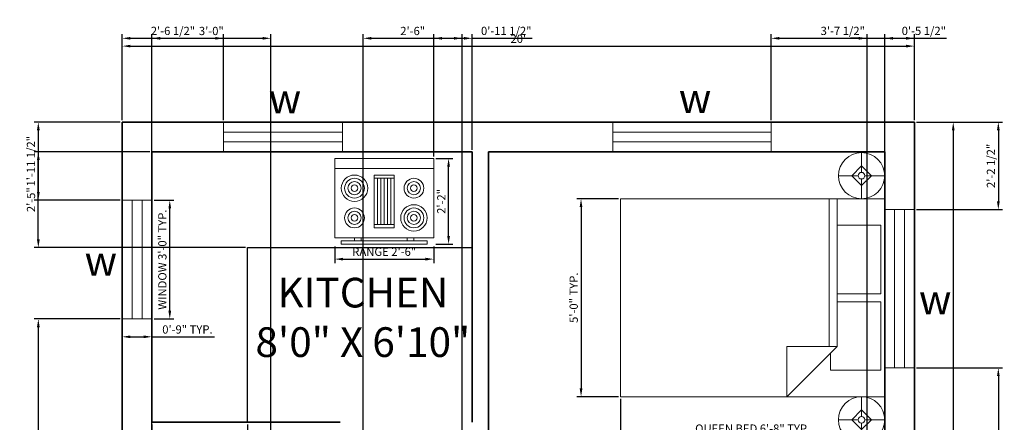
# Model space of a CAD drawing. Units: inches. Extents: x 3796 to 4094, y 4410 to 4948.
# Tile 3 of 3: x 3796 to 4094, y 4826 to 4948. Entities that reach past the tile are written whole.
import ezdxf

# ---------------------------------------------------------------- set-up
doc = ezdxf.new("R2010")
doc.units = ezdxf.units.IN
for name, color, linetype, lineweight in [('A-ANNO-DIMS', 2, 'Continuous', 18), ('A-ANNO-TEXT', 7, 'Continuous', 18), ('A-AREA-IDEN', 7, 'Continuous', 25), ('A-EQPM', 9, 'Continuous', 18), ('A-FLOR-CASE', 8, 'Continuous', 25), ('A-FURN', 8, 'Continuous', 18), ('A-GLAZ', 4, 'Continuous', 18), ('A-WALL', 7, 'Continuous', 35)]:
    doc.layers.add(name, color=color, linetype=linetype, lineweight=lineweight)
doc.styles.get("Standard").update_dxf_attribs({"font": 'arial.ttf'})
doc.dimstyles.new('ISO-25', dxfattribs={"dimtxt": 2.5, "dimasz": 2.5, "dimexe": 1.25, "dimexo": 0.625, "dimtad": 1, "dimdec": 0, "dimlunit": 3, "dimtxsty": 'Standard', "dimcen": 2.5, "dimadec": 0, "dimazin": 0, "dimtfac": 1, "dimtdec": 0, "dimtmove": 0, "dimatfit": 3, "dimfxl": 1, "dimarcsym": 0})

# ---------------------------------------------------------------- blocks, each defined once
blk = doc.blocks.new('*D1')
at = {"layer": 'A-ANNO-DIMS', "color": 0, "lineweight": -2, "transparency": 16777216}
for p, q in [((3826.76, 4917.18), (3826.76, 4940.86)), ((4066.76, 4917.18), (4066.76, 4940.86)), ((3829.26, 4939.61), (4064.26, 4939.61))]:
    blk.add_line(p, q, dxfattribs=at)
at = {"layer": 'A-ANNO-DIMS', "color": 0, "transparency": 16777216}
for points in [[(3829.26, 4940.03), (3829.26, 4939.19), (3826.76, 4939.61)], [(4064.26, 4940.03), (4064.26, 4939.19), (4066.76, 4939.61)]]:
    blk.add_solid(points, dxfattribs=at)
at = {"layer": 'Defpoints', "color": 0, "transparency": 16777216}
for p in [(4066.76, 4939.61), (3826.76, 4916.55), (4066.76, 4916.55)]:
    blk.add_point(p, dxfattribs=at)
at = {"layer": 'A-ANNO-DIMS', "color": 0, "transparency": 16777216, "insert": (3946.76, 4941.51), "char_height": 2.5, "attachment_point": 5}
blk.add_mtext("20'", dxfattribs=at)
blk = doc.blocks.new('*D2')
at = {"layer": 'A-ANNO-DIMS', "color": 0, "lineweight": -2, "transparency": 16777216}
for p, q in [((4067.39, 4916.55), (4079.78, 4916.55)), ((4078.53, 4914.05), (4078.53, 4439.05)), ((4067.39, 4436.55), (4079.78, 4436.55))]:
    blk.add_line(p, q, dxfattribs=at)
at = {"layer": 'A-ANNO-DIMS', "color": 0, "transparency": 16777216}
for points in [[(4078.11, 4914.05), (4078.94, 4914.05), (4078.53, 4916.55)], [(4078.11, 4439.05), (4078.94, 4439.05), (4078.53, 4436.55)]]:
    blk.add_solid(points, dxfattribs=at)
at = {"layer": 'Defpoints', "color": 0, "transparency": 16777216}
for p in [(4066.76, 4916.55), (4066.76, 4436.55), (4078.53, 4436.55)]:
    blk.add_point(p, dxfattribs=at)
at = {"layer": 'A-ANNO-DIMS', "color": 0, "transparency": 16777216, "insert": (4076.62, 4676.55), "char_height": 2.5, "attachment_point": 5, "rotation": 90}
blk.add_mtext("40'", dxfattribs=at)
blk = doc.blocks.new('Range-Oven - 30 in top')
for p, q in [((0, -3), (30, -3)), ((12, -6), (18, -6)), ((13, -20), (13, -6)), ((14, -6), (14, -20)), ((15, -20), (15, -6)), ((16, -6), (16, -20)), ((17, -20), (17, -6)), ((18, -20), (12, -20)), ((6, -24), (6, -25)), ((8, -25), (8, -24)), ((22, -25), (22, -24)), ((24, -24), (24, -25))]:
    blk.add_line(p, q)
for points in [[(0, -24), (0, 0), (30, 0), (30, -24)], [(12, -21), (12, -5), (18, -5), (18, -21)], [(2, -26), (2, -25), (28, -25), (28, -26)]]:
    blk.add_lwpolyline(points, close=True)
for centre, radius in [((6, -9), 4), ((6, -9), 3), ((6, -9), 2), ((6, -9), 1), ((24, -9), 3), ((24, -9), 2), ((24, -9), 1), ((24, -18), 4), ((6, -18), 3), ((6, -18), 2), ((6, -18), 1), ((24, -18), 3), ((24, -18), 2), ((24, -18), 1)]:
    blk.add_circle(centre, radius)
blk = doc.blocks.new('Bed - Queen')
for p, q in [((0, -80.00003), (0, 0)), ((0, 0), (59.99999, 0)), ((59.99999, 0), (59.99999, -80.00003)), ((7.99999, -1.2), (28.79998, -1.2)), ((7.99999, -14.4), (7.99999, -1.2)), ((28.79998, -1.2), (28.79998, -14.4)), ((31.19999, -1.2), (51.99999, -1.2)), ((31.19999, -14.4), (31.19999, -1.2)), ((51.99999, -1.2), (51.99999, -16.4)), ((0, -14.4), (44.8, -14.4)), ((59.99999, -29.6), (44.8, -14.4)), ((44.8, -14.4), (44.8, -29.6)), ((44.8, -16.8), (0, -16.8)), ((51.99999, -16.4), (46.79936, -16.4)), ((44.8, -29.6), (59.99999, -29.6)), ((59.99999, -80.00003), (0, -80.00003))]:
    blk.add_line(p, q)
blk = doc.blocks.new('Lamp - Table')
for p, q in [((0, 7), (0, 1)), ((0, 3), (-3, 0)), ((3, 0), (0, 3)), ((-1, 0), (-7, 0)), ((-3, 0), (0, -3)), ((0, -3), (3, 0)), ((1, 0), (7, 0)), ((0, -1), (0, -7))]:
    blk.add_line(p, q)
for radius in [7, 1]:
    blk.add_circle((0, 0), radius)
blk = doc.blocks.new('WIN-48IN')
for p, q in [((0, 48), (0, 0)), ((9, 48), (0, 48)), ((3, 48), (3, 0)), ((6, 0), (6, 48)), ((9, 0), (9, 48)), ((0, 0), (9, 0))]:
    blk.add_line(p, q)
blk = doc.blocks.new('WIN-36IN')
for p, q in [((9, 36), (0, 36)), ((0, 36), (0, 24)), ((3, 24), (3, 36)), ((6, 24), (6, 36)), ((9, 24), (9, 36)), ((0, 24), (0, 0)), ((3, 24), (3, 0)), ((6, 0), (6, 24)), ((9, 0), (9, 24)), ((0, 0), (9, 0))]:
    blk.add_line(p, q)
blk = doc.blocks.new('*D13')
at = {"layer": 'A-ANNO-DIMS', "color": 0, "lineweight": -2, "transparency": 16777216}
for p, q in [((3836.39, 4892.88), (3842.41, 4892.88)), ((3841.16, 4859.38), (3841.16, 4890.38)), ((3836.39, 4856.88), (3842.41, 4856.88))]:
    blk.add_line(p, q, dxfattribs=at)
at = {"layer": 'A-ANNO-DIMS', "color": 0, "transparency": 16777216}
for points in [[(3840.75, 4890.38), (3841.58, 4890.38), (3841.16, 4892.88)], [(3840.75, 4859.38), (3841.58, 4859.38), (3841.16, 4856.88)]]:
    blk.add_solid(points, dxfattribs=at)
at = {"layer": 'Defpoints', "color": 0, "transparency": 16777216}
for p in [(3835.76, 4892.88), (3841.16, 4892.88), (3835.76, 4856.88)]:
    blk.add_point(p, dxfattribs=at)
at = {"layer": 'A-ANNO-DIMS', "color": 0, "transparency": 16777216, "insert": (3839.24, 4874.88), "char_height": 2.5, "attachment_point": 5, "rotation": 90}
blk.add_mtext('WINDOW 3\'-0" TYP.', dxfattribs=at)
blk = doc.blocks.new('*D14')
at = {"layer": 'A-ANNO-DIMS', "color": 0, "lineweight": -2, "transparency": 16777216}
for p, q in [((3826.76, 4856.25), (3826.76, 4850.23)), ((3835.76, 4856.25), (3835.76, 4850.23)), ((3829.26, 4851.48), (3833.26, 4851.48)), ((3835.76, 4851.48), (3854.75, 4851.48))]:
    blk.add_line(p, q, dxfattribs=at)
at = {"layer": 'A-ANNO-DIMS', "color": 0, "transparency": 16777216}
for points in [[(3829.26, 4851.89), (3829.26, 4851.06), (3826.76, 4851.48)], [(3833.26, 4851.89), (3833.26, 4851.06), (3835.76, 4851.48)]]:
    blk.add_solid(points, dxfattribs=at)
at = {"layer": 'Defpoints', "color": 0, "transparency": 16777216}
for p in [(3826.76, 4856.88), (3835.76, 4856.88), (3835.76, 4851.48)]:
    blk.add_point(p, dxfattribs=at)
at = {"layer": 'A-ANNO-DIMS', "color": 0, "transparency": 16777216, "insert": (3846.51, 4853.38), "char_height": 2.5, "attachment_point": 5}
blk.add_mtext('0\'-9" TYP.', dxfattribs=at)
blk = doc.blocks.new('*D15')
at = {"layer": 'A-ANNO-DIMS', "color": 0, "lineweight": -2, "transparency": 16777216}
for p, q in [((3977.76, 4832.71), (3977.76, 4820.08)), ((4057.76, 4832.71), (4057.76, 4820.08)), ((3980.26, 4821.33), (4055.26, 4821.33))]:
    blk.add_line(p, q, dxfattribs=at)
at = {"layer": 'A-ANNO-DIMS', "color": 0, "transparency": 16777216}
for points in [[(3980.26, 4821.75), (3980.26, 4820.92), (3977.76, 4821.33)], [(4055.26, 4821.75), (4055.26, 4820.92), (4057.76, 4821.33)]]:
    blk.add_solid(points, dxfattribs=at)
at = {"layer": 'Defpoints', "color": 0, "transparency": 16777216}
for p in [(3977.76, 4833.33), (4057.76, 4833.33), (4057.76, 4821.33)]:
    blk.add_point(p, dxfattribs=at)
at = {"layer": 'A-ANNO-DIMS', "color": 0, "transparency": 16777216, "insert": (4017.76, 4823.33), "char_height": 2.5, "attachment_point": 5}
blk.add_mtext('QUEEN BED 6\'-8" TYP.', dxfattribs=at)
blk = doc.blocks.new('*D16')
at = {"layer": 'A-ANNO-DIMS', "color": 0, "lineweight": -2, "transparency": 16777216}
for p, q in [((3977.14, 4893.33), (3964.51, 4893.33)), ((3965.76, 4890.83), (3965.76, 4835.83)), ((3977.14, 4833.33), (3964.51, 4833.33))]:
    blk.add_line(p, q, dxfattribs=at)
at = {"layer": 'A-ANNO-DIMS', "color": 0, "transparency": 16777216}
for points in [[(3965.35, 4890.83), (3966.18, 4890.83), (3965.76, 4893.33)], [(3965.35, 4835.83), (3966.18, 4835.83), (3965.76, 4833.33)]]:
    blk.add_solid(points, dxfattribs=at)
at = {"layer": 'Defpoints', "color": 0, "transparency": 16777216}
for p in [(3977.76, 4893.33), (3965.76, 4833.33), (3977.76, 4833.33)]:
    blk.add_point(p, dxfattribs=at)
at = {"layer": 'A-ANNO-DIMS', "color": 0, "transparency": 16777216, "insert": (3963.86, 4863.33), "char_height": 2.5, "attachment_point": 5, "rotation": 90}
blk.add_mtext('5\'-0" TYP.', dxfattribs=at)
blk = doc.blocks.new('*D21')
at = {"layer": 'A-ANNO-DIMS', "color": 0, "lineweight": -2, "transparency": 16777216}
for p, q in [((3891.13, 4878.9), (3891.13, 4873.78)), ((3921.13, 4878.9), (3921.13, 4873.78)), ((3893.63, 4875.03), (3918.63, 4875.03))]:
    blk.add_line(p, q, dxfattribs=at)
at = {"layer": 'A-ANNO-DIMS', "color": 0, "transparency": 16777216}
for points in [[(3893.63, 4875.44), (3893.63, 4874.61), (3891.13, 4875.03)], [(3918.63, 4875.44), (3918.63, 4874.61), (3921.13, 4875.03)]]:
    blk.add_solid(points, dxfattribs=at)
at = {"layer": 'Defpoints', "color": 0, "transparency": 16777216}
for p in [(3891.13, 4879.53), (3921.13, 4879.53), (3921.13, 4875.03)]:
    blk.add_point(p, dxfattribs=at)
at = {"layer": 'A-ANNO-DIMS', "color": 0, "transparency": 16777216, "insert": (3906.13, 4876.94), "char_height": 2.5, "attachment_point": 5}
blk.add_mtext('RANGE 2\'-6"', dxfattribs=at)
blk = doc.blocks.new('*D22')
at = {"layer": 'A-ANNO-DIMS', "color": 0, "lineweight": -2, "transparency": 16777216}
for p, q in [((3921.76, 4905.53), (3926.88, 4905.53)), ((3925.63, 4882.03), (3925.63, 4903.03)), ((3921.76, 4879.53), (3926.88, 4879.53))]:
    blk.add_line(p, q, dxfattribs=at)
at = {"layer": 'A-ANNO-DIMS', "color": 0, "transparency": 16777216}
for points in [[(3925.22, 4903.03), (3926.05, 4903.03), (3925.63, 4905.53)], [(3925.22, 4882.03), (3926.05, 4882.03), (3925.63, 4879.53)]]:
    blk.add_solid(points, dxfattribs=at)
at = {"layer": 'Defpoints', "color": 0, "transparency": 16777216}
for p in [(3921.13, 4905.53), (3925.63, 4905.53), (3921.13, 4879.53)]:
    blk.add_point(p, dxfattribs=at)
at = {"layer": 'A-ANNO-DIMS', "color": 0, "transparency": 16777216, "insert": (3923.75, 4892.53), "char_height": 2.5, "attachment_point": 5, "rotation": 90}
blk.add_mtext('2\'-2"', dxfattribs=at)
blk = doc.blocks.new('*D31')
at = {"layer": 'A-ANNO-DIMS', "color": 0, "lineweight": -2, "transparency": 16777216}
for p, q in [((3835.76, 4482.18), (3835.76, 4943.23)), ((3871.76, 4490.18), (3871.76, 4943.23)), ((3838.26, 4941.98), (3869.26, 4941.98))]:
    blk.add_line(p, q, dxfattribs=at)
at = {"layer": 'A-ANNO-DIMS', "color": 0, "transparency": 16777216}
for points in [[(3838.26, 4942.39), (3838.26, 4941.56), (3835.76, 4941.98)], [(3869.26, 4942.39), (3869.26, 4941.56), (3871.76, 4941.98)]]:
    blk.add_solid(points, dxfattribs=at)
at = {"layer": 'Defpoints', "color": 0, "transparency": 16777216}
for p in [(3871.76, 4941.98), (3871.76, 4489.55), (3835.76, 4481.55)]:
    blk.add_point(p, dxfattribs=at)
at = {"layer": 'A-ANNO-DIMS', "color": 0, "transparency": 16777216, "insert": (3853.76, 4943.88), "char_height": 2.5, "attachment_point": 5}
blk.add_mtext('3\'-0"', dxfattribs=at)
blk = doc.blocks.new('*D34')
at = {"layer": 'A-ANNO-DIMS', "color": 0, "lineweight": -2, "transparency": 16777216}
for p, q in [((3899.76, 4580.18), (3899.76, 4943.23)), ((3929.76, 4580.18), (3929.76, 4943.23)), ((3902.26, 4941.98), (3927.26, 4941.98))]:
    blk.add_line(p, q, dxfattribs=at)
at = {"layer": 'A-ANNO-DIMS', "color": 0, "transparency": 16777216}
for points in [[(3902.26, 4942.39), (3902.26, 4941.56), (3899.76, 4941.98)], [(3927.26, 4942.39), (3927.26, 4941.56), (3929.76, 4941.98)]]:
    blk.add_solid(points, dxfattribs=at)
at = {"layer": 'Defpoints', "color": 0, "transparency": 16777216}
for p in [(3929.76, 4941.98), (3899.76, 4579.55), (3929.76, 4579.55)]:
    blk.add_point(p, dxfattribs=at)
at = {"layer": 'A-ANNO-DIMS', "color": 0, "transparency": 16777216, "insert": (3914.76, 4943.88), "char_height": 2.5, "attachment_point": 5}
blk.add_mtext('2\'-6"', dxfattribs=at)
blk = doc.blocks.new('*D35')
at = {"layer": 'A-ANNO-DIMS', "color": 0, "lineweight": -2, "transparency": 16777216}
for p, q in [((3826.76, 4917.18), (3826.76, 4943.23)), ((3857.49, 4917.18), (3857.49, 4943.23)), ((3829.26, 4941.98), (3854.99, 4941.98))]:
    blk.add_line(p, q, dxfattribs=at)
at = {"layer": 'A-ANNO-DIMS', "color": 0, "transparency": 16777216}
for points in [[(3829.26, 4942.39), (3829.26, 4941.56), (3826.76, 4941.98)], [(3854.99, 4942.39), (3854.99, 4941.56), (3857.49, 4941.98)]]:
    blk.add_solid(points, dxfattribs=at)
at = {"layer": 'Defpoints', "color": 0, "transparency": 16777216}
for p in [(3857.49, 4941.98), (3826.76, 4916.55), (3857.49, 4916.55)]:
    blk.add_point(p, dxfattribs=at)
at = {"layer": 'A-ANNO-DIMS', "color": 0, "transparency": 16777216, "insert": (3842.13, 4943.9), "char_height": 2.5, "attachment_point": 5}
blk.add_mtext('2\'-6 1/2"', dxfattribs=at)
blk = doc.blocks.new('*D36')
at = {"layer": 'A-ANNO-DIMS', "color": 0, "lineweight": -2, "transparency": 16777216}
for p, q in [((4023.35, 4917.17), (4023.35, 4943.23)), ((4066.76, 4917.18), (4066.76, 4943.23)), ((4025.85, 4941.98), (4064.26, 4941.98))]:
    blk.add_line(p, q, dxfattribs=at)
at = {"layer": 'A-ANNO-DIMS', "color": 0, "transparency": 16777216}
for points in [[(4025.85, 4942.39), (4025.85, 4941.56), (4023.35, 4941.98)], [(4064.26, 4942.39), (4064.26, 4941.56), (4066.76, 4941.98)]]:
    blk.add_solid(points, dxfattribs=at)
at = {"layer": 'Defpoints', "color": 0, "transparency": 16777216}
for p in [(4066.76, 4941.98), (4023.35, 4916.54), (4066.76, 4916.55)]:
    blk.add_point(p, dxfattribs=at)
at = {"layer": 'A-ANNO-DIMS', "color": 0, "transparency": 16777216, "insert": (4045.06, 4943.9), "char_height": 2.5, "attachment_point": 5}
blk.add_mtext('3\'-7 1/2"', dxfattribs=at)
blk = doc.blocks.new('*D37')
at = {"layer": 'A-ANNO-DIMS', "color": 0, "lineweight": -2, "transparency": 16777216}
for p, q in [((3826.14, 4916.55), (3800.09, 4916.55)), ((3801.34, 4914.05), (3801.34, 4895.38)), ((3826.14, 4892.88), (3800.09, 4892.88))]:
    blk.add_line(p, q, dxfattribs=at)
at = {"layer": 'A-ANNO-DIMS', "color": 0, "transparency": 16777216}
for points in [[(3800.92, 4914.05), (3801.76, 4914.05), (3801.34, 4916.55)], [(3800.92, 4895.38), (3801.76, 4895.38), (3801.34, 4892.88)]]:
    blk.add_solid(points, dxfattribs=at)
at = {"layer": 'Defpoints', "color": 0, "transparency": 16777216}
for p in [(3826.76, 4916.55), (3801.34, 4892.88), (3826.76, 4892.88)]:
    blk.add_point(p, dxfattribs=at)
at = {"layer": 'A-ANNO-DIMS', "color": 0, "transparency": 16777216, "insert": (3799.42, 4904.72), "char_height": 2.5, "attachment_point": 5, "rotation": 90}
blk.add_mtext('1\'-11 1/2"', dxfattribs=at)
blk = doc.blocks.new('*D38')
at = {"layer": 'A-ANNO-DIMS', "color": 0, "lineweight": -2, "transparency": 16777216}
for p, q in [((3826.14, 4856.88), (3800.09, 4856.88)), ((3801.34, 4854.38), (3801.34, 4727.05)), ((3826.14, 4724.55), (3800.09, 4724.55))]:
    blk.add_line(p, q, dxfattribs=at)
at = {"layer": 'A-ANNO-DIMS', "color": 0, "transparency": 16777216}
for points in [[(3800.92, 4854.38), (3801.76, 4854.38), (3801.34, 4856.88)], [(3800.92, 4727.05), (3801.76, 4727.05), (3801.34, 4724.55)]]:
    blk.add_solid(points, dxfattribs=at)
at = {"layer": 'Defpoints', "color": 0, "transparency": 16777216}
for p in [(3826.76, 4856.88), (3801.34, 4724.55), (3826.76, 4724.55)]:
    blk.add_point(p, dxfattribs=at)
at = {"layer": 'A-ANNO-DIMS', "color": 0, "transparency": 16777216, "insert": (3799.42, 4790.72), "char_height": 2.5, "attachment_point": 5, "rotation": 90}
blk.add_mtext('11\'-0 1/2"', dxfattribs=at)
blk = doc.blocks.new('*D40')
at = {"layer": 'A-ANNO-DIMS', "color": 0, "lineweight": -2, "transparency": 16777216}
for p, q in [((4067.39, 4916.55), (4093.44, 4916.55)), ((4092.19, 4914.05), (4092.19, 4892.55)), ((4067.39, 4890.05), (4093.44, 4890.05))]:
    blk.add_line(p, q, dxfattribs=at)
at = {"layer": 'A-ANNO-DIMS', "color": 0, "transparency": 16777216}
for points in [[(4091.77, 4914.05), (4092.61, 4914.05), (4092.19, 4916.55)], [(4091.77, 4892.55), (4092.61, 4892.55), (4092.19, 4890.05)]]:
    blk.add_solid(points, dxfattribs=at)
at = {"layer": 'Defpoints', "color": 0, "transparency": 16777216}
for p in [(4066.76, 4916.55), (4066.76, 4890.05), (4092.19, 4890.05)]:
    blk.add_point(p, dxfattribs=at)
at = {"layer": 'A-ANNO-DIMS', "color": 0, "transparency": 16777216, "insert": (4090.27, 4903.3), "char_height": 2.5, "attachment_point": 5, "rotation": 90}
blk.add_mtext('2\'-2 1/2"', dxfattribs=at)
blk = doc.blocks.new('*D41')
at = {"layer": 'A-ANNO-DIMS', "color": 0, "lineweight": -2, "transparency": 16777216}
for p, q in [((4067.39, 4842.05), (4093.44, 4842.05)), ((4092.19, 4839.55), (4092.19, 4718.53)), ((4067.39, 4716.03), (4093.44, 4716.03))]:
    blk.add_line(p, q, dxfattribs=at)
at = {"layer": 'A-ANNO-DIMS', "color": 0, "transparency": 16777216}
for points in [[(4091.77, 4839.55), (4092.61, 4839.55), (4092.19, 4842.05)], [(4091.77, 4718.53), (4092.61, 4718.53), (4092.19, 4716.03)]]:
    blk.add_solid(points, dxfattribs=at)
at = {"layer": 'Defpoints', "color": 0, "transparency": 16777216}
for p in [(4066.76, 4842.05), (4066.76, 4716.03), (4092.19, 4716.03)]:
    blk.add_point(p, dxfattribs=at)
at = {"layer": 'A-ANNO-DIMS', "color": 0, "transparency": 16777216, "insert": (4090.29, 4779.04), "char_height": 2.5, "attachment_point": 5, "rotation": 90}
blk.add_mtext('10\'-6"', dxfattribs=at)
blk = doc.blocks.new('*D45')
at = {"layer": 'A-ANNO-DIMS', "color": 0, "lineweight": -2, "transparency": 16777216}
for p, q in [((3835.76, 4824.93), (3835.76, 4409.83)), ((3864.76, 4824.93), (3864.76, 4409.83)), ((3862.26, 4411.08), (3838.26, 4411.08))]:
    blk.add_line(p, q, dxfattribs=at)
at = {"layer": 'A-ANNO-DIMS', "color": 0, "transparency": 16777216}
for points in [[(3838.26, 4411.49), (3838.26, 4410.66), (3835.76, 4411.08)], [(3862.26, 4411.49), (3862.26, 4410.66), (3864.76, 4411.08)]]:
    blk.add_solid(points, dxfattribs=at)
at = {"layer": 'Defpoints', "color": 0, "transparency": 16777216}
for p in [(3835.76, 4825.55), (3864.76, 4825.55), (3835.76, 4411.08)]:
    blk.add_point(p, dxfattribs=at)
at = {"layer": 'A-ANNO-DIMS', "color": 0, "transparency": 16777216, "insert": (3850.26, 4412.98), "char_height": 2.5, "attachment_point": 5}
blk.add_mtext('2\'-5"', dxfattribs=at)
blk = doc.blocks.new('*D46')
at = {"layer": 'A-ANNO-DIMS', "color": 0, "lineweight": -2, "transparency": 16777216}
for p, q in [((3835.14, 4907.55), (3800.09, 4907.55)), ((3801.34, 4881.05), (3801.34, 4905.05)), ((3864.14, 4878.55), (3800.09, 4878.55))]:
    blk.add_line(p, q, dxfattribs=at)
at = {"layer": 'A-ANNO-DIMS', "color": 0, "transparency": 16777216}
for points in [[(3800.92, 4905.05), (3801.76, 4905.05), (3801.34, 4907.55)], [(3800.92, 4881.05), (3801.76, 4881.05), (3801.34, 4878.55)]]:
    blk.add_solid(points, dxfattribs=at)
at = {"layer": 'Defpoints', "color": 0, "transparency": 16777216}
for p in [(3801.34, 4907.55), (3835.76, 4907.55), (3864.76, 4878.55)]:
    blk.add_point(p, dxfattribs=at)
at = {"layer": 'A-ANNO-DIMS', "color": 0, "transparency": 16777216, "insert": (3799.44, 4893.05), "char_height": 2.5, "attachment_point": 5, "rotation": 90}
blk.add_mtext('2\'-5"', dxfattribs=at)
blk = doc.blocks.new('*D47')
at = {"layer": 'A-ANNO-DIMS', "color": 0, "lineweight": -2, "transparency": 16777216}
for p, q in [((3921.13, 4906.15), (3921.13, 4943.23)), ((3932.76, 4908.18), (3932.76, 4943.23)), ((3923.63, 4941.98), (3930.26, 4941.98)), ((3932.76, 4941.98), (3950.93, 4941.98))]:
    blk.add_line(p, q, dxfattribs=at)
at = {"layer": 'A-ANNO-DIMS', "color": 0, "transparency": 16777216}
for points in [[(3923.63, 4942.39), (3923.63, 4941.56), (3921.13, 4941.98)], [(3930.26, 4942.39), (3930.26, 4941.56), (3932.76, 4941.98)]]:
    blk.add_solid(points, dxfattribs=at)
at = {"layer": 'Defpoints', "color": 0, "transparency": 16777216}
for p in [(3932.76, 4941.98), (3932.76, 4907.55), (3921.13, 4905.53)]:
    blk.add_point(p, dxfattribs=at)
at = {"layer": 'A-ANNO-DIMS', "color": 0, "transparency": 16777216, "insert": (3943.1, 4943.9), "char_height": 2.5, "attachment_point": 5}
blk.add_mtext('0\'-11 1/2"', dxfattribs=at)
blk = doc.blocks.new('*D48')
at = {"layer": 'A-ANNO-DIMS', "color": 0, "lineweight": -2, "transparency": 16777216}
for p, q in [((4052.41, 4640.18), (4052.41, 4943.23)), ((4057.76, 4640.18), (4057.76, 4943.23)), ((4049.91, 4941.98), (4047.41, 4941.98)), ((4052.41, 4941.98), (4057.76, 4941.98)), ((4060.26, 4941.98), (4076.49, 4941.98))]:
    blk.add_line(p, q, dxfattribs=at)
at = {"layer": 'A-ANNO-DIMS', "color": 0, "transparency": 16777216}
for points in [[(4049.91, 4942.39), (4049.91, 4941.56), (4052.41, 4941.98)], [(4060.26, 4942.39), (4060.26, 4941.56), (4057.76, 4941.98)]]:
    blk.add_solid(points, dxfattribs=at)
at = {"layer": 'Defpoints', "color": 0, "transparency": 16777216}
for p in [(4057.76, 4941.98), (4052.41, 4639.55), (4057.76, 4639.55)]:
    blk.add_point(p, dxfattribs=at)
at = {"layer": 'A-ANNO-DIMS', "color": 0, "transparency": 16777216, "insert": (4069.62, 4943.9), "char_height": 2.5, "attachment_point": 5}
blk.add_mtext('0\'-5 1/2"', dxfattribs=at)

msp = doc.modelspace()

# ---------------------------------------------------------------- linework, layer by layer
at = {"layer": 'A-FLOR-CASE'}
for p, q in [((3864.76, 4878.55), (3932.76, 4878.55)), ((3864.76, 4825.55), (3864.76, 4878.55))]:
    msp.add_line(p, q, dxfattribs=at)
at = {"layer": 'A-WALL'}
for p, q in [((3826.76, 4916.55), (4066.76, 4916.55)), ((3826.76, 4436.55), (3826.76, 4916.55)), ((4066.76, 4916.55), (4066.76, 4436.55)), ((3835.76, 4907.55), (3932.76, 4907.55)), ((3835.76, 4825.55), (3835.76, 4907.55)), ((3932.76, 4907.55), (3932.76, 4825.55)), ((3937.76, 4907.55), (3937.76, 4817.55)), ((3937.76, 4907.55), (4057.76, 4907.55)), ((3937.76, 4817.55), (3937.76, 4907.55)), ((4057.76, 4907.55), (4057.76, 4781.55)), ((3835.76, 4825.55), (3892.75, 4825.55))]:
    msp.add_line(p, q, dxfattribs=at)

# ---------------------------------------------------------------- block references
at = {"layer": 'A-EQPM'}
msp.add_blockref('Range-Oven - 30 in top', (3891.13, 4905.53), dxfattribs=at)
at = {"layer": 'A-FURN', "rotation": 270}
for name, p in [('Lamp - Table', (4050.76, 4900.33)), ('Bed - Queen', (4057.76, 4893.33)), ('Lamp - Table', (4050.76, 4826.33))]:
    msp.add_blockref(name, p, dxfattribs=at)
at = {"layer": 'A-GLAZ'}
for name, p, rotation in [('WIN-36IN', (3857.49, 4916.55), 270.0000000000029), ('WIN-48IN', (4023.35, 4907.54), 89.99999999999916)]:
    msp.add_blockref(name, p, dxfattribs=dict(at, rotation=rotation))
for name, p in [('WIN-36IN', (3826.76, 4856.88)), ('WIN-48IN', (4057.76, 4842.05))]:
    msp.add_blockref(name, p, dxfattribs=at)

# ---------------------------------------------------------------- texts
at = {"layer": 'A-ANNO-TEXT', "char_height": 9, "attachment_point": 1}
for insert in [(3846.57, 4928.21), (3970.83, 4928.34), (3790.8, 4879.06), (4043.58, 4867.33)]:
    msp.add_mtext_dynamic_manual_height_columns('\\pxqc;w', width=58.9432, gutter_width=12.5, heights=[0], dxfattribs=dict(at, insert=insert))
at = {"layer": 'A-AREA-IDEN', "insert": (3862.85, 4869.37), "char_height": 9, "attachment_point": 1}
msp.add_mtext_dynamic_manual_height_columns('\\pxqc;KITCHEN\\P8\'0" X 6\'10"', width=73.619, gutter_width=12.5, heights=[0], dxfattribs=at)

# ---------------------------------------------------------------- dimensions: what is measured, and where the dimension line sits
at = {"layer": 'A-ANNO-DIMS'}
for base, p1, p2, override, picture, middle in [((3857.49, 4941.98), (3826.76, 4916.55), (3857.49, 4916.55), {"dimdec": 1, "dimlfac": 1, "dimrnd": 0, "dimzin": 1, "dimdsep": 46, "dimlunit": 4, "dimfrac": 2}, '*D35', (3842.13, 4943.9)), ((3932.76, 4941.98), (3921.13, 4905.53), (3932.76, 4907.55), {"dimdec": 1, "dimlfac": 1, "dimrnd": 0, "dimzin": 1, "dimdsep": 46, "dimlunit": 4, "dimfrac": 2}, '*D47', (3943.1, 4943.9)), ((4066.76, 4941.98), (4023.35, 4916.54), (4066.76, 4916.55), {"dimdec": 1, "dimlfac": 1, "dimrnd": 0, "dimzin": 1, "dimdsep": 46, "dimlunit": 4, "dimfrac": 2}, '*D36', (4045.06, 4943.9)), ((4057.7642, 4941.9774), (4052.4081, 4639.5524), (4057.7642, 4639.5524), {"dimdec": 1, "dimlfac": 1, "dimrnd": 0, "dimzin": 1, "dimdsep": 46, "dimlunit": 4, "dimfrac": 2}, '*D48', (4069.6247, 4943.8951)), ((4066.76, 4939.61), (3826.76, 4916.55), (4066.76, 4916.55), {"dimclrd": 0, "dimclre": 0, "dimclrt": 0}, '*D1', (3946.76, 4941.51)), ((3871.76, 4941.98), (3835.76, 4481.55), (3871.76, 4489.55), {"dimdec": 1, "dimlfac": 1, "dimrnd": 0, "dimzin": 1, "dimdsep": 46, "dimlunit": 4, "dimfrac": 2}, '*D31', (3853.76, 4943.88)), ((3929.76, 4941.98), (3899.76, 4579.55), (3929.76, 4579.55), {"dimdec": 1, "dimlfac": 1, "dimrnd": 0, "dimzin": 1, "dimdsep": 46, "dimlunit": 4, "dimfrac": 2}, '*D34', (3914.76, 4943.88)), ((3835.76, 4411.08), (3864.76, 4825.55), (3835.76, 4825.55), {"dimdec": 1, "dimlfac": 1, "dimrnd": 0, "dimzin": 1, "dimdsep": 46, "dimlunit": 4, "dimfrac": 2}, '*D45', (3850.26, 4412.98))]:
    dim = msp.add_linear_dim(base=base, p1=p1, p2=p2, dimstyle='ISO-25', override=override, dxfattribs=at)
    dim.commit()
    dim.dimension.update_dxf_attribs({"geometry": picture, "text_midpoint": middle})
for base, p1, p2, override, picture, middle in [((3801.34, 4892.88), (3826.76, 4916.55), (3826.76, 4892.88), {"dimdec": 1, "dimlfac": 1, "dimrnd": 0, "dimzin": 1, "dimdsep": 46, "dimlunit": 4, "dimfrac": 2}, '*D37', (3799.42, 4904.72)), ((4078.53, 4436.55), (4066.76, 4916.55), (4066.76, 4436.55), {"dimclrd": 0, "dimclre": 0, "dimclrt": 0}, '*D2', (4076.62, 4676.55)), ((4092.19, 4890.05), (4066.76, 4916.55), (4066.76, 4890.05), {"dimdec": 1, "dimlfac": 1, "dimrnd": 0, "dimzin": 1, "dimdsep": 46, "dimlunit": 4, "dimfrac": 2}, '*D40', (4090.27, 4903.3)), ((3801.34, 4907.55), (3864.76, 4878.55), (3835.76, 4907.55), {"dimdec": 1, "dimlfac": 1, "dimrnd": 0, "dimzin": 1, "dimdsep": 46, "dimlunit": 4, "dimfrac": 2}, '*D46', (3799.44, 4893.05)), ((3925.63, 4905.53), (3921.13, 4879.53), (3921.13, 4905.53), {"dimdec": 1, "dimlfac": 1, "dimrnd": 0, "dimzin": 1, "dimdsep": 46, "dimlunit": 4, "dimfrac": 2}, '*D22', (3923.75, 4892.53)), ((3801.34, 4724.55), (3826.76, 4856.88), (3826.76, 4724.55), {"dimdec": 1, "dimlfac": 1, "dimrnd": 0, "dimzin": 1, "dimdsep": 46, "dimlunit": 4, "dimfrac": 2}, '*D38', (3799.42, 4790.72)), ((4092.19, 4716.03), (4066.76, 4842.05), (4066.76, 4716.03), {"dimdec": 1, "dimlfac": 1, "dimrnd": 0, "dimzin": 1, "dimdsep": 46, "dimlunit": 4, "dimfrac": 2}, '*D41', (4090.29, 4779.04))]:
    dim = msp.add_linear_dim(base=base, p1=p1, p2=p2, angle=90, dimstyle='ISO-25', override=override, dxfattribs=at)
    dim.commit()
    dim.dimension.update_dxf_attribs({"geometry": picture, "text_midpoint": middle})
for base, p1, p2, angle, text, picture, middle in [((3841.16, 4892.88), (3835.76, 4856.88), (3835.76, 4892.88), 90, 'WINDOW <> TYP.', '*D13', (3839.24, 4874.88)), ((3965.76, 4833.33), (3977.76, 4893.33), (3977.76, 4833.33), 270, '<> TYP.', '*D16', (3963.86, 4863.33))]:
    dim = msp.add_linear_dim(base=base, p1=p1, p2=p2, angle=angle, text=text, dimstyle='ISO-25', override={"dimdec": 1, "dimlfac": 1, "dimrnd": 0, "dimzin": 1, "dimdsep": 46, "dimlunit": 4, "dimfrac": 2}, dxfattribs=at)
    dim.commit()
    dim.dimension.update_dxf_attribs({"geometry": picture, "text_midpoint": middle})
for base, p1, p2, text, picture, middle in [((3921.13, 4875.03), (3891.13, 4879.53), (3921.13, 4879.53), 'RANGE <>', '*D21', (3906.13, 4876.94)), ((3835.76, 4851.48), (3826.76, 4856.88), (3835.76, 4856.88), '<> TYP.', '*D14', (3846.51, 4853.38)), ((4057.76, 4821.33), (3977.76, 4833.33), (4057.76, 4833.33), 'QUEEN BED <> TYP.', '*D15', (4017.76, 4823.33))]:
    dim = msp.add_linear_dim(base=base, p1=p1, p2=p2, text=text, dimstyle='ISO-25', override={"dimdec": 1, "dimlfac": 1, "dimrnd": 0, "dimzin": 1, "dimdsep": 46, "dimlunit": 4, "dimfrac": 2}, dxfattribs=at)
    dim.commit()
    dim.dimension.update_dxf_attribs({"geometry": picture, "text_midpoint": middle})

doc.saveas('drawing.dxf')
